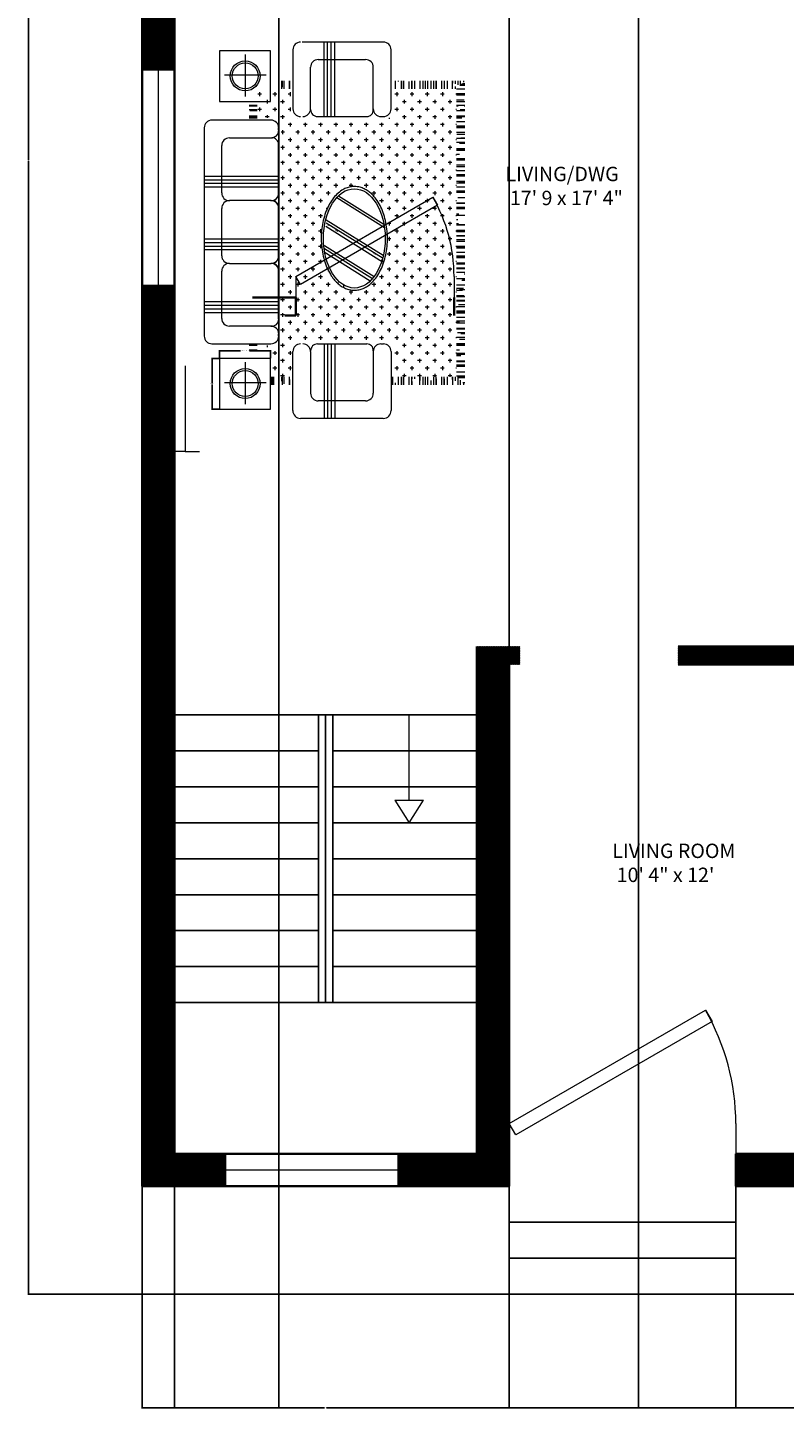
# Model space of a CAD drawing. Units: inches. Extents: x -19 to 404, y -21 to 673.
# Tile 1 of 3: x -19 to 191, y -21 to 363. Entities that reach past the tile are written whole.
import ezdxf

# ---------------------------------------------------------------- set-up
doc = ezdxf.new("R2010")
doc.units = ezdxf.units.IN
doc.header["$MEASUREMENT"] = 0
for name, color, linetype, lineweight in [('A-ANNO-DIMS', 2, 'Continuous', 18), ('A-ANNO-SYMB', 7, 'Continuous', 18), ('A-AREA-IDEN', 7, 'Continuous', 18), ('A-FLOR-STRS', 7, 'Continuous', 25), ('A-FURN', 8, 'Continuous', 18), ('A-FURN-PATT', 8, 'Continuous', 13), ('A-WALL', 7, 'Continuous', 35), ('doors', 40, 'Continuous', 18), ('window', 30, 'Continuous', 18)]:
    doc.layers.add(name, color=color, linetype=linetype, lineweight=lineweight)
doc.layers.add('A-WALL-PATT', color=244, linetype='Continuous', lineweight=13, true_color=0x991b1e)
doc.styles.get("Standard").update_dxf_attribs({"font": 'arial.ttf'})
doc.dimstyles.get("Standard").update_dxf_attribs({"dimtxt": 0.18, "dimasz": 0.18, "dimexe": 0.18, "dimexo": 0.0625, "dimgap": 0.09, "dimtad": 0, "dimtih": 1, "dimtoh": 1, "dimdec": 4, "dimzin": 0, "dimdsep": 46, "dimtxsty": 'Standard', "dimcen": 0.09, "dimadec": 0, "dimazin": 0, "dimtfac": 1, "dimtdec": 4, "dimtofl": 0, "dimtmove": 0, "dimatfit": 3, "dimfxl": 1, "dimtolj": 1, "dimtzin": 0, "dimarcsym": 0})
pattern_1 = [(45, (-13642.13922, -42713.83606), (-0.08838834765, 0.08838834765), [])]

# ---------------------------------------------------------------- blocks, each defined once
blk = doc.blocks.new('*U5')
for p, q in [((0, 0), (0, -100)), ((750, 0), (750, -100))]:
    blk.add_line(p, q)
blk.add_lwpolyline([(0, 0), (649.5, 375), (671.4, 337.1), (21.9, -37.9)], close=True)
blk.add_arc((0, 0), 750, 0, 30)
blk = doc.blocks.new('LAMP-END-TABLE')
for p, q in [((14.11, 14.11), (0, 14.11)), ((0, 14.11), (0, 0)), ((7.16, 1.4), (7.16, 13.04)), ((14.11, 0), (14.11, 14.11)), ((12.97, 7.3), (1.33, 7.3)), ((0, 0), (14.11, 0))]:
    blk.add_line(p, q)
for radius in [4.16, 3.6]:
    blk.add_circle((7.1, 7.11), radius)
blk = doc.blocks.new('*D19')
at = {"layer": 'A-ANNO-DIMS', "color": 0, "lineweight": -2, "transparency": 16777216}
for p, q in [((34.21, 270.93), (34.21, 273.17)), ((34.39, 272.99), (40.01, 272.99)), ((48.14, 272.99), (42.52, 272.99)), ((48.32, 270.93), (48.32, 273.17))]:
    blk.add_line(p, q, dxfattribs=at)
at = {"layer": 'A-ANNO-DIMS', "color": 0, "transparency": 16777216}
for points in [[(34.39, 273.02), (34.39, 272.96), (34.21, 272.99)], [(48.14, 273.02), (48.14, 272.96), (48.32, 272.99)]]:
    blk.add_solid(points, dxfattribs=at)
at = {"layer": 'Defpoints', "color": 0, "transparency": 16777216}
for p in [(48.32, 272.99), (34.21, 270.87), (48.32, 270.87)]:
    blk.add_point(p, dxfattribs=at)
at = {"layer": 'A-ANNO-DIMS', "color": 0, "transparency": 16777216, "insert": (41.27, 272.99), "char_height": 0.18, "attachment_point": 5}
blk.add_mtext('\\A1;END TABLE 14 TYP.', dxfattribs=at)
blk = doc.blocks.new('*D20')
at = {"layer": 'A-ANNO-DIMS', "color": 0, "lineweight": -2, "transparency": 16777216}
for p, q in [((34.15, 270.87), (31.92, 270.87)), ((32.1, 270.69), (32.1, 264)), ((32.1, 256.94), (32.1, 263.64)), ((34.15, 256.76), (31.92, 256.76))]:
    blk.add_line(p, q, dxfattribs=at)
at = {"layer": 'A-ANNO-DIMS', "color": 0, "transparency": 16777216}
for points in [[(32.07, 270.69), (32.13, 270.69), (32.1, 270.87)], [(32.07, 256.94), (32.13, 256.94), (32.1, 256.76)]]:
    blk.add_solid(points, dxfattribs=at)
at = {"layer": 'Defpoints', "color": 0, "transparency": 16777216}
for p in [(32.1, 270.87), (34.21, 270.87), (34.21, 256.76)]:
    blk.add_point(p, dxfattribs=at)
at = {"layer": 'A-ANNO-DIMS', "color": 0, "transparency": 16777216, "insert": (32.1, 263.82), "char_height": 0.18, "attachment_point": 5}
blk.add_mtext('\\A1;14 TYP.', dxfattribs=at)
blk = doc.blocks.new('*D26')
at = {"layer": 'A-ANNO-DIMS', "color": 0, "lineweight": -2, "transparency": 16777216}
for p, q in [((12.59, 640.82), (-19.13, 640.82)), ((-18.95, 640.64), (-18.95, 326)), ((-18.95, 11), (-18.95, 325.64)), ((114.59, 10.82), (-19.13, 10.82))]:
    blk.add_line(p, q, dxfattribs=at)
at = {"layer": 'A-ANNO-DIMS', "color": 0, "transparency": 16777216}
for points in [[(-18.98, 640.64), (-18.92, 640.64), (-18.95, 640.82)], [(-18.98, 11), (-18.92, 11), (-18.95, 10.82)]]:
    blk.add_solid(points, dxfattribs=at)
at = {"layer": 'Defpoints', "color": 0, "transparency": 16777216}
for p in [(12.65, 640.82), (-18.95, 10.82), (114.65, 10.82)]:
    blk.add_point(p, dxfattribs=at)
at = {"layer": 'A-ANNO-DIMS', "color": 0, "transparency": 16777216, "insert": (-18.95, 325.82), "char_height": 0.18, "attachment_point": 5}
blk.add_mtext('\\A1;630', dxfattribs=at)
blk = doc.blocks.new('*D27')
at = {"layer": 'A-ANNO-DIMS', "color": 0, "lineweight": -2, "transparency": 16777216}
for p, q in [((372.71, 40.82), (404.42, 40.82)), ((404.24, 40.64), (404.24, 26)), ((404.24, 11), (404.24, 25.64)), ((177.71, 10.82), (404.42, 10.82))]:
    blk.add_line(p, q, dxfattribs=at)
at = {"layer": 'A-ANNO-DIMS', "color": 0, "transparency": 16777216}
for points in [[(404.21, 40.64), (404.27, 40.64), (404.24, 40.82)], [(404.21, 11), (404.27, 11), (404.24, 10.82)]]:
    blk.add_solid(points, dxfattribs=at)
at = {"layer": 'Defpoints', "color": 0, "transparency": 16777216}
for p in [(372.65, 40.82), (177.65, 10.82), (404.24, 10.82)]:
    blk.add_point(p, dxfattribs=at)
at = {"layer": 'A-ANNO-DIMS', "color": 0, "transparency": 16777216, "insert": (404.24, 25.82), "char_height": 0.18, "attachment_point": 5}
blk.add_mtext('\\A1;30', dxfattribs=at)
blk = doc.blocks.new('*D28')
at = {"layer": 'A-ANNO-DIMS', "color": 0, "lineweight": -2, "transparency": 16777216}
for p, q in [((12.65, 40.76), (12.65, -20.95)), ((114.65, 40.76), (114.65, -20.95)), ((12.83, -20.77), (63.37, -20.77)), ((114.47, -20.77), (63.93, -20.77))]:
    blk.add_line(p, q, dxfattribs=at)
at = {"layer": 'A-ANNO-DIMS', "color": 0, "transparency": 16777216}
for points in [[(12.83, -20.74), (12.83, -20.8), (12.65, -20.77)], [(114.47, -20.74), (114.47, -20.8), (114.65, -20.77)]]:
    blk.add_solid(points, dxfattribs=at)
at = {"layer": 'Defpoints', "color": 0, "transparency": 16777216}
for p in [(12.65, 40.82), (114.65, 40.82), (114.65, -20.77)]:
    blk.add_point(p, dxfattribs=at)
at = {"layer": 'A-ANNO-DIMS', "color": 0, "transparency": 16777216, "insert": (63.65, -20.77), "char_height": 0.18, "attachment_point": 5}
blk.add_mtext('\\A1;102', dxfattribs=at)
blk = doc.blocks.new('*D29')
at = {"layer": 'A-ANNO-DIMS', "color": 0, "lineweight": -2, "transparency": 16777216}
for p, q in [((114.65, 10.76), (114.65, -20.95)), ((177.65, 10.76), (177.65, -20.95)), ((114.83, -20.77), (145.93, -20.77)), ((177.47, -20.77), (146.37, -20.77))]:
    blk.add_line(p, q, dxfattribs=at)
at = {"layer": 'A-ANNO-DIMS', "color": 0, "transparency": 16777216}
for points in [[(114.83, -20.74), (114.83, -20.8), (114.65, -20.77)], [(177.47, -20.74), (177.47, -20.8), (177.65, -20.77)]]:
    blk.add_solid(points, dxfattribs=at)
at = {"layer": 'Defpoints', "color": 0, "transparency": 16777216}
for p in [(114.65, 10.82), (177.65, 10.82), (177.65, -20.77)]:
    blk.add_point(p, dxfattribs=at)
at = {"layer": 'A-ANNO-DIMS', "color": 0, "transparency": 16777216, "insert": (146.15, -20.77), "char_height": 0.18, "attachment_point": 5}
blk.add_mtext('\\A1;63', dxfattribs=at)
blk = doc.blocks.new('*D30')
at = {"layer": 'A-ANNO-DIMS', "color": 0, "lineweight": -2, "transparency": 16777216}
for p, q in [((239.65, 49.76), (239.65, -20.95)), ((177.65, 10.76), (177.65, -20.95)), ((177.83, -20.77), (208.43, -20.77)), ((239.47, -20.77), (208.87, -20.77))]:
    blk.add_line(p, q, dxfattribs=at)
at = {"layer": 'A-ANNO-DIMS', "color": 0, "transparency": 16777216}
for points in [[(177.83, -20.74), (177.83, -20.8), (177.65, -20.77)], [(239.47, -20.74), (239.47, -20.8), (239.65, -20.77)]]:
    blk.add_solid(points, dxfattribs=at)
at = {"layer": 'Defpoints', "color": 0, "transparency": 16777216}
for p in [(239.65, 49.82), (177.65, 10.82), (239.65, -20.77)]:
    blk.add_point(p, dxfattribs=at)
at = {"layer": 'A-ANNO-DIMS', "color": 0, "transparency": 16777216, "insert": (208.65, -20.77), "char_height": 0.18, "attachment_point": 5}
blk.add_mtext('\\A1;62', dxfattribs=at)
blk = doc.blocks.new('*D38')
at = {"layer": 'A-ANNO-DIMS', "color": 0, "lineweight": -2, "transparency": 16777216}
for p, q in [((21.65, 386.76), (21.65, -20.95)), ((50.65, 386.76), (50.65, -20.95)), ((21.83, -20.77), (35.93, -20.77)), ((50.47, -20.77), (36.37, -20.77))]:
    blk.add_line(p, q, dxfattribs=at)
at = {"layer": 'A-ANNO-DIMS', "color": 0, "transparency": 16777216}
for points in [[(21.83, -20.74), (21.83, -20.8), (21.65, -20.77)], [(50.47, -20.74), (50.47, -20.8), (50.65, -20.77)]]:
    blk.add_solid(points, dxfattribs=at)
at = {"layer": 'Defpoints', "color": 0, "transparency": 16777216}
for p in [(21.65, 386.82), (50.65, 386.82), (50.65, -20.77)]:
    blk.add_point(p, dxfattribs=at)
at = {"layer": 'A-ANNO-DIMS', "color": 0, "transparency": 16777216, "insert": (36.15, -20.77), "char_height": 0.18, "attachment_point": 5}
blk.add_mtext('\\A1;29', dxfattribs=at)
blk = doc.blocks.new('*D40')
at = {"layer": 'A-ANNO-DIMS', "color": 0, "lineweight": -2, "transparency": 16777216}
for p, q in [((114.65, 381.76), (114.65, -20.95)), ((150.65, 381.76), (150.65, -20.95)), ((114.83, -20.77), (132.43, -20.77)), ((150.47, -20.77), (132.87, -20.77))]:
    blk.add_line(p, q, dxfattribs=at)
at = {"layer": 'A-ANNO-DIMS', "color": 0, "transparency": 16777216}
for points in [[(114.83, -20.74), (114.83, -20.8), (114.65, -20.77)], [(150.47, -20.74), (150.47, -20.8), (150.65, -20.77)]]:
    blk.add_solid(points, dxfattribs=at)
at = {"layer": 'Defpoints', "color": 0, "transparency": 16777216}
for p in [(114.65, 381.82), (150.65, 381.82), (150.65, -20.77)]:
    blk.add_point(p, dxfattribs=at)
at = {"layer": 'A-ANNO-DIMS', "color": 0, "transparency": 16777216, "insert": (132.65, -20.77), "char_height": 0.18, "attachment_point": 5}
blk.add_mtext('\\A1;36', dxfattribs=at)

msp = doc.modelspace()

# ---------------------------------------------------------------- hatches: boundary and pattern name
at = {"layer": 'A-FURN-PATT'}
h = msp.add_hatch(dxfattribs=at)
h.set_pattern_fill('AR-RROOF', color=256, scale=2.507942, angle=630, style=0)
h.set_pattern_definition([(180, (292.9002, 622.0426), (-4.965726, 2.257148), [33.85722, -4.5143, 11.28574, -2.25715]), (180, (289.8982, 623.171), (2.257148, 3.002007), [6.771445, -0.74486, 13.54289, -1.69286]), (180, (291.7716, 623.9611), (-11.7371705, 1.5122893), [18.057185, -3.16001, 9.028593, -2.25715])])
h.paths.add_polyline_path([(42.42, 272.94), (42.42, 274.92), (44.68, 274.92), (44.68, 272.94)])
h.paths.add_polyline_path([(100.06, 265.77), (100.06, 345.77), (102.32, 348.03), (102.32, 263.51)])
h.paths.add_polyline_path([(42.42, 337.1), (42.42, 342.33), (44.68, 342.04), (44.68, 337.1)])
h = msp.add_hatch(dxfattribs=at)
h.set_pattern_fill('CROSS', color=256, scale=9.404784, angle=540, style=0)
h.set_pattern_definition([(270, (292.9002, 622.0426), (-2.116076, -2.116076), [1.058038, -3.174115]), (180, (293.4292, 621.5135), (-2.116076, 2.116076), [1.058038, -3.174115])])
h.paths.add_polyline_path([(82.55, 265.77), (82.33, 273.68), (82.19, 275.31), (55.75, 275.45), (54.13, 274.5), (54.22, 265.77), (48.32, 265.77), (48.32, 272.94), (44.68, 272.94), (44.68, 274.33), (51.01, 274.5), (51.28, 336.22), (50.33, 337.72), (44.68, 337.64), (44.68, 343), (45.08, 345.77), (54, 345.77), (53.85, 339.21), (55.75, 337.44), (78.53, 337.04), (82.19, 337.99), (82.44, 345.77), (100.06, 345.77), (100.06, 265.77)])
h.paths.add_polyline_path([(80.02, 302.31), (79.89, 312.35), (75.28, 317.91), (73.24, 318.72), (70.67, 318.72), (68.77, 318.32), (66.19, 317.1), (65.11, 314.52), (63.62, 311.53), (62.94, 308.28), (62.53, 304.34), (64.02, 296.07), (67.41, 291.32), (72.84, 290.37), (75.95, 291.86), (78.67, 295.8)], flags=16)
edge = h.paths.add_edge_path(flags=0)
edge.add_line((78.81, 298.97), (64.01, 307.87))
edge.add_ellipse((86.9, 304.4), major_axis=(-16.37, 16.37), ratio=1, start_angle=35.8767, end_angle=36.3651, ccw=False)
edge.add_line((64.04, 308.07), (78.86, 299.16))
edge.add_ellipse((56.31, 304.4), major_axis=(16.37, 16.37), ratio=1, start_angle=301.4454, end_angle=301.9202, ccw=False)
edge.add_line((78.81, 298.97), (78.81, 298.97))
edge.add_ellipse((63.86, 302.58), major_axis=(10.88, 10.88), ratio=1, start_angle=301.4399, end_angle=301.4562)
edge.add_line((78.81, 298.98), (78.81, 298.98))
edge.add_line((78.81, 298.98), (78.81, 298.98))
edge.add_line((78.81, 298.98), (78.81, 298.98))
edge.add_line((78.81, 298.98), (78.81, 298.98))
edge.add_line((78.81, 298.98), (78.81, 298.98))
edge.add_ellipse((63.86, 302.58), major_axis=(-10.88, 10.88), ratio=1, start_angle=211.4399, end_angle=211.4562, ccw=False)
h = msp.add_hatch(dxfattribs=at)
h.set_pattern_fill('AR-RROOF', color=256, scale=2.507942, angle=540, style=0)
h.set_pattern_definition([(270, (292.9002, 622.0426), (-2.257148, -4.965726), [33.85722, -4.5143, 11.28574, -2.25715]), (270, (291.7716, 619.0406), (-3.002007, 2.257148), [6.771445, -0.74486, 13.54289, -1.69286]), (270, (290.9816, 620.914), (-1.5122893, -11.7371705), [18.057185, -3.16001, 9.028593, -2.25715])])
h.paths.add_polyline_path([(48.32, 263.51), (48.32, 265.77), (54.57, 265.77), (54.57, 263.51)])
h.paths.add_polyline_path([(81.86, 263.51), (81.86, 265.77), (100.06, 265.77), (102.32, 263.51)])
h.paths.add_polyline_path([(81.86, 345.77), (81.86, 348.03), (102.32, 348.03), (100.06, 345.77)])
h.paths.add_polyline_path([(51.06, 345.77), (51.35, 348.03), (54.57, 348.03), (54.57, 345.77)])
at = {"layer": 'A-WALL-PATT'}
h = msp.add_hatch(dxfattribs=at)
h.set_pattern_fill('ANSI31', color=256)
h.set_pattern_definition(pattern_1)
h.paths.add_polyline_path([(45.83, 640.82), (12.65, 640.82), (12.65, 610.17), (17.15, 610.17), (21.65, 610.17), (21.65, 631.82), (45.83, 631.82)])
h.paths.add_polyline_path([(21.65, 550.17), (12.65, 550.17), (12.65, 468.55), (17.15, 468.55), (21.65, 468.55), (21.65, 482.82), (153.65, 482.82), (153.65, 386.82), (150.65, 386.82), (150.65, 381.82), (158.65, 381.82), (158.65, 490.82), (153.65, 490.82), (153.65, 487.82), (21.65, 487.82)])
h.paths.add_polyline_path([(21.65, 420.55), (12.65, 420.55), (12.65, 351.11), (17.15, 351.11), (21.65, 351.11), (21.65, 381.82), (114.65, 381.82), (114.65, 386.82), (21.65, 386.82)])
h.paths.add_polyline_path([(21.65, 291.11), (12.65, 291.11), (12.65, 40.82), (35.81, 40.82), (35.81, 49.82), (21.65, 49.82)])
h.paths.add_polyline_path([(114.65, 185.82), (117.65, 185.82), (117.65, 190.82), (114.65, 190.82), (113.65, 190.82), (110.65, 190.82), (105.65, 190.82), (105.65, 49.82), (83.81, 49.82), (83.81, 40.82), (114.65, 40.82)])
h = msp.add_hatch(dxfattribs=at)
h.set_pattern_fill('ANSI31', color=256)
h.set_pattern_definition(pattern_1)
h.paths.add_polyline_path([(195.39, 49.82), (177.65, 49.82), (177.65, 40.82), (195.39, 40.82)])
h.paths.add_polyline_path([(276.02, 49.82), (239.65, 49.82), (239.65, 146.82), (234.65, 146.82), (234.65, 49.82), (219.39, 49.82), (219.39, 40.82), (276.02, 40.82)])
h.paths.add_polyline_path([(372.65, 87.37), (363.65, 87.37), (363.65, 49.82), (324.02, 49.82), (324.02, 40.82), (372.65, 40.82)])
h.paths.add_polyline_path([(372.65, 280.5), (363.65, 280.5), (363.65, 243.82), (271.65, 243.82), (271.65, 238.82), (274.65, 238.82), (274.65, 190.82), (161.65, 190.82), (161.65, 185.82), (234.65, 185.82), (234.65, 182.82), (239.65, 182.82), (239.65, 185.82), (282.65, 185.82), (282.65, 190.82), (279.65, 190.82), (279.65, 238.82), (363.65, 238.82), (363.65, 225.27), (368.15, 225.27), (372.65, 225.27)])
h.paths.add_polyline_path([(372.65, 201.27), (363.65, 201.27), (363.65, 190.82), (311.65, 190.82), (311.65, 185.82), (363.65, 185.82), (363.65, 135.37), (368.15, 135.37), (372.65, 135.37)])
h.paths.add_polyline_path([(372.65, 383.98), (363.65, 383.98), (363.65, 327.82), (239.65, 327.82), (239.65, 330.82), (234.65, 330.82), (234.65, 327.82), (234.65, 238.82), (242.65, 238.82), (242.65, 243.82), (239.65, 243.82), (239.65, 322.82), (363.65, 322.82), (363.65, 304.5), (368.15, 304.5), (372.65, 304.5)])

# ---------------------------------------------------------------- linework, layer by layer
at = {"layer": 'A-ANNO-SYMB'}
for p, q in [((24.62, 268.77), (24.62, 244.99)), ((24.62, 244.99), (20.62, 244.99)), ((24.62, 244.99), (28.62, 244.99)), ((86.9, 148.04), (86.9, 171.82)), ((82.9, 148.04), (86.9, 141.82)), ((82.9, 148.04), (90.9, 148.04)), ((86.9, 141.82), (90.9, 148.04))]:
    msp.add_line(p, q, dxfattribs=at)
at = {"layer": 'A-FLOR-STRS'}
for p, q in [((21.65, 171.82), (105.65, 171.82)), ((61.65, 171.82), (61.65, 91.82)), ((63.65, 171.82), (63.65, 91.82)), ((65.65, 171.82), (65.65, 91.82)), ((21.65, 161.82), (61.65, 161.82)), ((65.65, 161.82), (105.65, 161.82)), ((21.65, 151.82), (61.65, 151.82)), ((65.65, 151.82), (105.65, 151.82)), ((21.65, 141.82), (61.65, 141.82)), ((65.65, 141.82), (105.65, 141.82)), ((21.65, 131.82), (61.65, 131.82)), ((65.65, 131.82), (105.65, 131.82)), ((21.65, 121.82), (61.65, 121.82)), ((65.65, 121.82), (105.65, 121.82)), ((21.65, 111.82), (61.65, 111.82)), ((65.65, 111.82), (105.65, 111.82)), ((21.65, 101.82), (61.65, 101.82)), ((65.65, 101.82), (105.65, 101.82)), ((21.65, 49.82), (21.65, 91.82)), ((21.65, 91.82), (105.65, 91.82)), ((114.65, 40.82), (114.65, 30.82)), ((177.65, 30.82), (177.65, 40.82)), ((114.65, 30.82), (177.65, 30.82)), ((114.65, 30.82), (114.65, 20.82)), ((177.65, 20.82), (177.65, 30.82)), ((177.65, 30.82), (177.65, 20.82)), ((114.65, 20.82), (177.65, 20.82)), ((114.65, 10.82), (114.65, 20.82)), ((177.65, 20.82), (177.65, 10.82)), ((177.65, 10.82), (114.65, 10.82))]:
    msp.add_line(p, q, dxfattribs=at)
at = {"layer": 'A-FURN'}
for p, q in [((80.14, 358.71), (57.12, 358.71)), ((63.22, 338.14), (63.22, 358.77)), ((64.21, 338.14), (64.21, 358.77)), ((65.21, 338.14), (65.21, 358.77)), ((66.2, 338.14), (66.2, 358.77)), ((54.57, 356.64), (54.57, 340.23)), ((61.61, 353.92), (74.78, 353.92)), ((81.86, 340.23), (81.86, 356.64)), ((59.48, 340.23), (59.48, 351.78)), ((76.92, 340.04), (76.91, 351.78)), ((61.42, 338.1), (75.12, 338.1)), ((79.04, 338.1), (79.72, 338.1)), ((29.93, 334.96), (29.93, 277.06)), ((48.48, 337.1), (32.07, 337.1)), ((50.61, 334.28), (50.61, 335.06)), ((36.93, 332.14), (48.48, 332.14)), ((50.61, 316.65), (50.61, 330.34)), ((34.79, 316.84), (34.79, 330)), ((50.57, 321.43), (29.93, 321.43)), ((50.57, 320.44), (29.93, 320.44)), ((50.57, 319.44), (29.93, 319.44)), ((50.57, 318.45), (29.93, 318.45)), ((48.48, 314.71), (36.93, 314.71)), ((66.77, 315.56), (80.01, 307.25)), ((67.27, 316.07), (79.86, 308.17)), ((34.79, 299.41), (34.79, 312.57)), ((50.61, 299.21), (50.61, 312.91)), ((63.74, 307.64), (79.51, 297.74)), ((63.85, 309.4), (79.63, 299.51)), ((63.85, 308.58), (79.63, 298.68)), ((50.57, 304), (29.93, 304)), ((50.57, 303), (29.93, 303)), ((50.57, 302.01), (29.93, 302.01)), ((50.57, 301.01), (29.93, 301.01)), ((63.27, 300.45), (76.08, 292.41)), ((63.38, 302.22), (77.12, 293.6)), ((63.38, 301.39), (76.68, 293.05)), ((36.93, 297.26), (48.48, 297.26)), ((34.79, 281.97), (34.79, 295.13)), ((50.61, 281.77), (50.61, 295.47)), ((50.57, 286.55), (29.93, 286.55)), ((50.57, 285.56), (29.93, 285.56)), ((50.57, 284.56), (29.93, 284.56)), ((50.57, 283.57), (29.93, 283.57)), ((48.48, 279.83), (36.93, 279.83)), ((50.61, 277.06), (50.61, 277.69)), ((32.07, 274.92), (48.48, 274.92)), ((54.57, 256.34), (54.57, 272.75)), ((59.48, 272.75), (59.48, 261.2)), ((61.42, 274.89), (75.12, 274.89)), ((63.22, 274.84), (63.22, 254.21)), ((64.21, 274.84), (64.21, 254.21)), ((65.21, 274.84), (65.21, 254.21)), ((66.2, 274.84), (66.2, 254.21)), ((76.92, 272.94), (76.91, 261.2)), ((79.04, 274.89), (79.72, 274.89)), ((81.86, 272.75), (81.86, 256.34)), ((74.78, 259.06), (61.61, 259.06)), ((56.66, 254.21), (79.68, 254.21))]:
    msp.add_line(p, q, dxfattribs=at)
for centre, radius, start, end in [((56.71, 356.64), 2.14, 90, 180), ((79.72, 356.64), 2.14, 0, 90), ((61.61, 351.78), 2.14, 90, 180), ((74.78, 351.78), 2.14, 0, 90), ((56.71, 340.23), 2.14, 180, 270), ((57.34, 340.23), 2.14, 270, 0), ((61.4, 340.02), 1.92, 179.3701, 270.6589), ((75.12, 339.89), 1.8, 270, 2.986), ((79.04, 340.23), 2.14, 180, 270), ((79.72, 340.23), 2.14, 270, 0), ((32.07, 334.96), 2.14, 90, 180), ((48.48, 334.96), 2.14, 0, 90), ((48.48, 334.28), 2.14, 270, 0), ((36.93, 330), 2.14, 90, 180), ((48.81, 330.34), 1.8, 0, 92.986), ((36.93, 316.84), 2.14, 180, 270), ((36.93, 312.57), 2.14, 90, 180), ((48.48, 316.84), 2.14, 270, 0), ((48.48, 312.57), 2.14, 0, 90), ((48.69, 316.63), 1.92, 269.3701, 0.6589), ((48.81, 312.91), 1.8, 0, 92.986), ((36.93, 299.41), 2.14, 180, 270), ((48.48, 299.4), 2.14, 270, 0), ((36.93, 295.13), 2.14, 90, 180), ((48.48, 295.13), 2.14, 0, 90), ((48.69, 299.19), 1.92, 269.3701, 0.6589), ((48.81, 295.47), 1.8, 0, 92.986), ((36.93, 281.97), 2.14, 180, 270), ((48.68, 281.76), 1.94, 264.1019, 0.4455), ((32.07, 277.06), 2.14, 180, 270), ((48.48, 277.69), 2.14, 0, 90), ((48.48, 277.06), 2.14, 270, 0), ((56.71, 272.75), 2.14, 90, 180), ((57.34, 272.75), 2.14, 0, 90), ((61.4, 272.96), 1.92, 89.3411, 180.6299), ((75.12, 273.09), 1.8, 357.014, 90), ((79.04, 272.75), 2.14, 90, 180), ((79.72, 272.75), 2.14, 0, 90), ((61.61, 261.2), 2.14, 180, 270), ((74.78, 261.2), 2.14, 270, 0), ((56.67, 256.34), 2.14, 180, 270), ((79.72, 256.34), 2.14, 270, 0)]:
    msp.add_arc(centre, radius, start, end, dxfattribs=at)
at = {"layer": 'A-FURN', "extrusion": (0, 0, -1)}
msp.add_ellipse((71.65, 304.22), major_axis=(0, 13.79), ratio=0.62186, start_param=4.712389, end_param=10.995574, dxfattribs=at)
at = {"layer": 'A-FURN'}
msp.add_open_spline([(71.65, 318.63), (71.92, 318.63), (72.19, 318.62), (72.74, 318.54), (73.01, 318.48), (73.65, 318.31), (74.03, 318.16), (74.76, 317.81), (75.12, 317.59), (75.81, 317.11), (76.15, 316.83), (76.79, 316.21), (77.1, 315.88), (77.8, 315), (78.18, 314.44), (78.87, 313.23), (79.18, 312.57), (79.73, 311.2), (79.96, 310.47), (80.36, 308.98), (80.51, 308.2), (80.74, 306.62), (80.81, 305.82), (80.87, 304.2), (80.85, 303.39), (80.74, 301.78), (80.63, 300.98), (80.35, 299.43), (80.16, 298.67), (79.72, 297.21), (79.45, 296.51), (78.86, 295.18), (78.52, 294.56), (77.78, 293.41), (77.38, 292.88), (76.52, 291.94), (76.06, 291.52), (75.21, 290.9), (74.83, 290.66), (74.04, 290.27), (73.63, 290.12), (72.81, 289.9), (72.39, 289.83), (71.55, 289.79), (71.13, 289.81), (70.29, 289.94), (69.88, 290.05), (69.07, 290.36), (68.68, 290.55), (67.91, 291.02), (67.54, 291.29), (66.83, 291.9), (66.49, 292.25), (65.84, 293), (65.53, 293.4), (64.88, 294.4), (64.54, 295), (63.94, 296.28), (63.67, 296.96), (63.21, 298.38), (63.02, 299.11), (62.72, 300.63), (62.61, 301.4), (62.47, 302.97), (62.44, 303.77), (62.46, 305.35), (62.52, 306.15), (62.7, 307.7), (62.84, 308.47), (63.19, 309.96), (63.4, 310.68), (63.9, 312.06), (64.19, 312.72), (64.83, 313.96), (65.18, 314.54), (65.95, 315.59), (66.37, 316.07), (67.25, 316.92), (67.71, 317.29), (68.56, 317.82), (68.94, 318.02), (69.7, 318.33), (70.1, 318.44), (70.88, 318.6), (71.26, 318.63), (71.65, 318.63)], degree=3, knots=[3.141593, 3.141593, 3.141593, 3.141593, 3.226917, 3.226917, 3.312242, 3.312242, 3.434267, 3.434267, 3.556292, 3.556292, 3.678317, 3.678317, 3.800342, 3.800342, 3.971574, 3.971574, 4.142806, 4.142806, 4.314038, 4.314038, 4.48527, 4.48527, 4.656502, 4.656502, 4.827734, 4.827734, 4.998965, 4.998965, 5.170197, 5.170197, 5.341429, 5.341429, 5.512661, 5.512661, 5.683893, 5.683893, 5.855125, 5.855125, 5.986691, 5.986691, 6.118257, 6.118257, 6.249823, 6.249823, 6.381389, 6.381389, 6.512955, 6.512955, 6.644521, 6.644521, 6.776087, 6.776087, 6.907652, 6.907652, 7.039218, 7.039218, 7.207016, 7.207016, 7.374813, 7.374813, 7.54261, 7.54261, 7.710407, 7.710407, 7.878205, 7.878205, 8.046002, 8.046002, 8.213799, 8.213799, 8.381596, 8.381596, 8.549393, 8.549393, 8.717191, 8.717191, 8.884988, 8.884988, 9.052785, 9.052785, 9.178207, 9.178207, 9.303629, 9.303629, 9.424778, 9.424778, 9.424778, 9.424778], dxfattribs=at)
at = {"layer": 'A-WALL'}
for p, q in [((21.65, 49.82), (21.65, 381.82)), ((43.36, 287.77), (55.36, 287.77)), ((48.36, 287.77), (51.36, 287.77)), ((55.36, 287.77), (51.36, 287.77)), ((52.36, 287.77), (55.36, 287.77)), ((55.36, 287.77), (55.36, 282.77)), ((99.36, 282.77), (99.36, 287.77)), ((52.36, 282.77), (55.36, 282.77)), ((52.36, 282.77), (55.36, 282.77)), ((105.65, 49.82), (105.65, 190.82)), ((161.65, 190.82), (274.65, 190.82)), ((114.65, 40.82), (114.65, 185.82)), ((161.65, 185.82), (234.65, 185.82)), ((105.65, 49.82), (21.65, 49.82)), ((234.65, 49.82), (177.65, 49.82)), ((177.65, 40.82), (177.65, 49.82))]:
    msp.add_line(p, q, dxfattribs=at)
msp.add_lwpolyline([(114.65, 40.82), (12.65, 40.82), (12.65, 640.82), (372.65, 640.82), (372.65, 40.82), (177.65, 40.82)], dxfattribs=at)
at = {"layer": 'window'}
for p, q in [((12.65, 351.11), (21.65, 351.11)), ((12.65, 291.11), (12.65, 351.11)), ((12.65, 351.11), (17.15, 351.11)), ((17.15, 351.11), (17.15, 291.11)), ((21.65, 351.11), (21.65, 291.11)), ((21.65, 291.11), (12.65, 291.11)), ((35.81, 49.82), (35.81, 40.82)), ((83.81, 49.82), (35.81, 49.82)), ((35.81, 49.82), (35.81, 45.32)), ((83.81, 40.82), (83.81, 49.82)), ((35.81, 45.32), (83.81, 45.32)), ((35.81, 40.82), (71.81, 40.82)), ((71.81, 40.82), (83.81, 40.82))]:
    msp.add_line(p, q, dxfattribs=at)

# ---------------------------------------------------------------- block references
at = {"layer": 'A-FURN'}
for p in [(34.21, 342.27), (34.21, 256.76)]:
    msp.add_blockref('LAMP-END-TABLE', p, dxfattribs=at)
at = {"layer": 'doors'}
for p, xscale, yscale, zscale in [((55.36, 293.63), 0.0586666666666683, 0.0586666666666683, 0.0586666666666683), ((114.65, 58.22), 0.0839999999999999, 0.0839999999999999, 0.0839999999999999)]:
    msp.add_blockref('*U5', p, dxfattribs=dict(at, xscale=xscale, yscale=yscale, zscale=zscale))

# ---------------------------------------------------------------- texts
at = {"layer": 'A-AREA-IDEN', "char_height": 4, "attachment_point": 1}
for s, insert in [('   LIVING/DWG\\P    17\' 9 x 17\' 4"', (109.98, 324.12)), ('  LIVING ROOM\\P   10\' 4" x 12\'', (140.88, 136))]:
    msp.add_mtext_dynamic_manual_height_columns(s, width=75.0771, gutter_width=1, heights=[0], dxfattribs=dict(at, insert=insert))

# ---------------------------------------------------------------- dimensions: what is measured, and where the dimension line sits
at = {"layer": 'A-ANNO-DIMS'}
for base, p1, p2, picture, middle in [((-18.95, 10.82), (12.65, 640.82), (114.65, 10.82), '*D26', (-18.95, 325.82)), ((404.24, 10.82), (372.65, 40.82), (177.65, 10.82), '*D27', (404.24, 25.82))]:
    dim = msp.add_linear_dim(base=base, p1=p1, p2=p2, angle=90, dimstyle='Standard', override={"dimdec": 0, "dimlfac": 1, "dimrnd": 0, "dimzin": 0, "dimdsep": 46, "dimlunit": 2}, dxfattribs=at)
    dim.commit()
    dim.dimension.update_dxf_attribs({"geometry": picture, "text_midpoint": middle})
for base, p1, p2, picture, middle in [((50.65, -20.77), (21.65, 386.82), (50.65, 386.82), '*D38', (36.15, -20.77)), ((150.65, -20.77), (114.65, 381.82), (150.65, 381.82), '*D40', (132.65, -20.77)), ((239.65, -20.77), (177.65, 10.82), (239.65, 49.82), '*D30', (208.65, -20.77)), ((114.65, -20.77), (12.65, 40.82), (114.65, 40.82), '*D28', (63.65, -20.77)), ((177.65, -20.77), (114.65, 10.82), (177.65, 10.82), '*D29', (146.15, -20.77))]:
    dim = msp.add_linear_dim(base=base, p1=p1, p2=p2, dimstyle='Standard', override={"dimdec": 0, "dimlfac": 1, "dimrnd": 0, "dimzin": 0, "dimdsep": 46, "dimlunit": 2}, dxfattribs=at)
    dim.commit()
    dim.dimension.update_dxf_attribs({"geometry": picture, "text_midpoint": middle})
dim = msp.add_linear_dim(base=(48.32, 272.99), p1=(34.21, 270.87), p2=(48.32, 270.87), text='END TABLE <> TYP.', dimstyle='Standard', override={"dimdec": 0, "dimlfac": 1, "dimrnd": 0, "dimzin": 0, "dimdsep": 46, "dimlunit": 2}, dxfattribs=at)
dim.commit()
dim.dimension.update_dxf_attribs({"geometry": '*D19', "text_midpoint": (41.27, 272.99)})
dim = msp.add_linear_dim(base=(32.1, 270.87), p1=(34.21, 256.76), p2=(34.21, 270.87), angle=90, text='<> TYP.', dimstyle='Standard', override={"dimdec": 0, "dimlfac": 1, "dimrnd": 0, "dimzin": 0, "dimdsep": 46, "dimlunit": 2}, dxfattribs=at)
dim.commit()
dim.dimension.update_dxf_attribs({"geometry": '*D20', "text_midpoint": (32.1, 263.82)})

doc.saveas('drawing.dxf')
